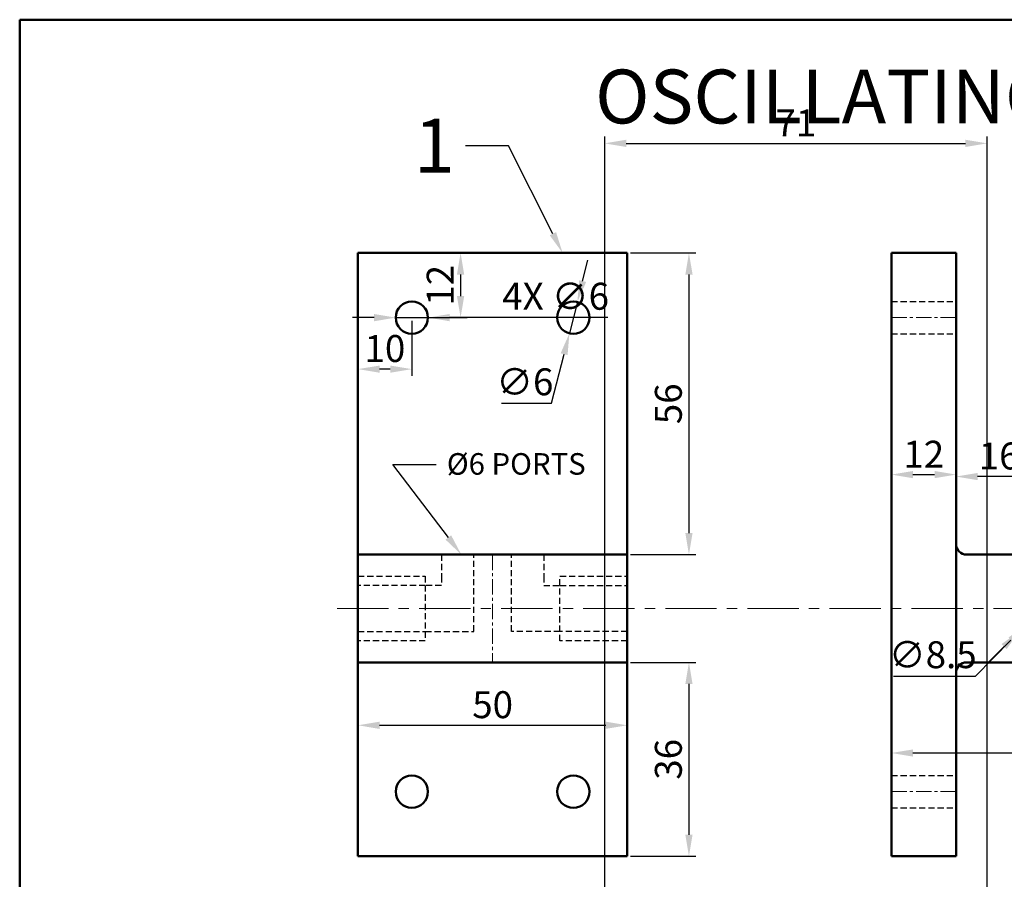
# Model space of a CAD drawing. Units: millimetres. Extents: x 24 to 508, y -182 to 223.
# Tile 2 of 6: x 24 to 207, y 63 to 223. Entities that reach past the tile are written whole.
import ezdxf
from ezdxf import colors
from ezdxf.entities.mleader import LeaderData, LeaderLine
from ezdxf.math import Vec2, Vec3

# ---------------------------------------------------------------- set-up
doc = ezdxf.new("R2010")
doc.units = ezdxf.units.MM
doc.header["$LTSCALE"] = 0.3
doc.linetypes.add('CENTER', pattern=[50.8, 31.75, -6.35, 6.35, -6.35])
doc.linetypes.add('DASHED', pattern=[19.05, 12.7, -6.35])
for name, color, linetype, lineweight in [('M-CNTR', 1, 'CENTER', 18), ('M-DIMS', 2, 'Continuous', 25), ('M-HIDN', 4, 'DASHED', 25), ('M-OUTL', 7, 'Continuous', 50), ('M-TEXT', 7, 'Continuous', 25)]:
    doc.layers.add(name, color=color, linetype=linetype, lineweight=lineweight)
doc.styles.get("Standard").update_dxf_attribs({"font": 'arial.ttf'})
doc.dimstyles.new('ISO-25', dxfattribs={"dimtxt": 5, "dimasz": 4, "dimexe": 1.25, "dimexo": 0.625, "dimtad": 1, "dimtoh": 1, "dimdec": 0, "dimtxsty": 'Standard', "dimcen": 2.5, "dimadec": 0, "dimazin": 0, "dimtfac": 1, "dimtdec": 0, "dimtmove": 0, "dimatfit": 3, "dimfxl": 1, "dimarcsym": 0})

# ---------------------------------------------------------------- blocks, each defined once
blk = doc.blocks.new('*D1')
at = {"layer": 'Defpoints', "color": 0, "ltscale": 0.3, "transparency": 16777216}
for p in [(136.55, 179.44), (136.55, 123.44), (148.01, 123.44)]:
    blk.add_point(p, dxfattribs=at)
at = {"layer": 'M-DIMS', "color": 0, "lineweight": -2, "ltscale": 0.3, "transparency": 16777216}
for p, q in [((137.17, 179.44), (149.26, 179.44)), ((148.01, 175.44), (148.01, 127.44)), ((137.17, 123.44), (149.26, 123.44))]:
    blk.add_line(p, q, dxfattribs=at)
at = {"layer": 'M-DIMS', "color": 0, "ltscale": 0.3, "transparency": 16777216}
for points in [[(147.34, 175.44), (148.68, 175.44), (148.01, 179.44)], [(147.34, 127.44), (148.68, 127.44), (148.01, 123.44)]]:
    blk.add_solid(points, dxfattribs=at)
at = {"layer": 'M-DIMS', "color": 0, "ltscale": 0.3, "transparency": 16777216, "insert": (144.83, 151.44), "char_height": 5, "attachment_point": 5, "rotation": 90}
blk.add_mtext('56', dxfattribs=at)
blk = doc.blocks.new('*D2')
at = {"layer": 'Defpoints', "color": 0, "ltscale": 0.3, "transparency": 16777216}
for p in [(136.55, 103.44), (136.55, 67.44), (148.01, 67.44)]:
    blk.add_point(p, dxfattribs=at)
at = {"layer": 'M-DIMS', "color": 0, "lineweight": -2, "ltscale": 0.3, "transparency": 16777216}
for p, q in [((137.17, 103.44), (149.26, 103.44)), ((148.01, 99.44), (148.01, 71.44)), ((137.17, 67.44), (149.26, 67.44))]:
    blk.add_line(p, q, dxfattribs=at)
at = {"layer": 'M-DIMS', "color": 0, "ltscale": 0.3, "transparency": 16777216}
for points in [[(147.34, 99.44), (148.68, 99.44), (148.01, 103.44)], [(147.34, 71.44), (148.68, 71.44), (148.01, 67.44)]]:
    blk.add_solid(points, dxfattribs=at)
at = {"layer": 'M-DIMS', "color": 0, "ltscale": 0.3, "transparency": 16777216, "insert": (144.83, 85.44), "char_height": 5, "attachment_point": 5, "rotation": 90}
blk.add_mtext('36', dxfattribs=at)
blk = doc.blocks.new('*D3')
at = {"layer": 'Defpoints', "color": 0, "ltscale": 0.3, "transparency": 16777216}
for p in [(86.55, 179.44), (96.55, 167.44), (105.6, 167.44)]:
    blk.add_point(p, dxfattribs=at)
at = {"layer": 'M-DIMS', "color": 0, "lineweight": -2, "ltscale": 0.3, "transparency": 16777216}
for p, q in [((87.17, 179.44), (106.85, 179.44)), ((105.6, 175.44), (105.6, 171.44)), ((97.17, 167.44), (106.85, 167.44))]:
    blk.add_line(p, q, dxfattribs=at)
at = {"layer": 'M-DIMS', "color": 0, "ltscale": 0.3, "transparency": 16777216}
for points in [[(104.93, 175.44), (106.27, 175.44), (105.6, 179.44)], [(104.93, 171.44), (106.27, 171.44), (105.6, 167.44)]]:
    blk.add_solid(points, dxfattribs=at)
at = {"layer": 'M-DIMS', "color": 0, "ltscale": 0.3, "transparency": 16777216, "insert": (102.46, 173.44), "char_height": 5, "attachment_point": 5, "rotation": 90}
blk.add_mtext('12', dxfattribs=at)
blk = doc.blocks.new('*D4')
at = {"layer": 'Defpoints', "color": 0, "ltscale": 0.3, "transparency": 16777216}
for p in [(86.55, 167.44), (96.55, 167.44), (86.55, 157.88)]:
    blk.add_point(p, dxfattribs=at)
at = {"layer": 'M-DIMS', "color": 0, "lineweight": -2, "ltscale": 0.3, "transparency": 16777216}
for p, q in [((86.55, 166.82), (86.55, 156.63)), ((96.55, 166.82), (96.55, 156.63)), ((92.55, 157.88), (90.55, 157.88))]:
    blk.add_line(p, q, dxfattribs=at)
at = {"layer": 'M-DIMS', "color": 0, "ltscale": 0.3, "transparency": 16777216}
for points in [[(90.55, 158.54), (90.55, 157.21), (86.55, 157.88)], [(92.55, 158.54), (92.55, 157.21), (96.55, 157.88)]]:
    blk.add_solid(points, dxfattribs=at)
at = {"layer": 'M-DIMS', "color": 0, "ltscale": 0.3, "transparency": 16777216, "insert": (91.55, 161.06), "char_height": 5, "attachment_point": 5}
blk.add_mtext('10', dxfattribs=at)
blk = doc.blocks.new('*D5')
at = {"layer": 'Defpoints', "color": 0, "ltscale": 0.3, "transparency": 16777216}
for p in [(127.29, 170.35), (125.81, 164.53)]:
    blk.add_point(p, dxfattribs=at)
at = {"layer": 'M-DIMS', "color": 0, "lineweight": -2, "ltscale": 0.3, "transparency": 16777216}
for p, q in [((128.27, 174.22), (129.26, 178.1)), ((127.29, 170.35), (125.81, 164.53)), ((122.51, 151.56), (124.82, 160.66)), ((113.17, 151.56), (122.51, 151.56))]:
    blk.add_line(p, q, dxfattribs=at)
at = {"layer": 'M-DIMS', "color": 0, "ltscale": 0.3, "transparency": 16777216}
for points in [[(127.63, 174.39), (128.92, 174.06), (127.29, 170.35)], [(124.18, 160.82), (125.47, 160.49), (125.81, 164.53)]]:
    blk.add_solid(points, dxfattribs=at)
at = {"layer": 'M-DIMS', "color": 0, "ltscale": 0.3, "transparency": 16777216, "insert": (117.53, 154.88), "char_height": 5, "attachment_point": 5}
blk.add_mtext('∅6', dxfattribs=at)
blk = doc.blocks.new('*D6')
at = {"layer": 'Defpoints', "color": 0, "ltscale": 0.3, "transparency": 16777216}
for p in [(86.55, 93.5), (136.55, 93.5), (136.55, 91.76)]:
    blk.add_point(p, dxfattribs=at)
at = {"layer": 'M-DIMS', "color": 0, "lineweight": -2, "ltscale": 0.3, "transparency": 16777216}
for p, q in [((86.55, 92.88), (86.55, 90.51)), ((90.55, 91.76), (132.55, 91.76)), ((136.55, 92.88), (136.55, 90.51))]:
    blk.add_line(p, q, dxfattribs=at)
at = {"layer": 'M-DIMS', "color": 0, "ltscale": 0.3, "transparency": 16777216}
for points in [[(90.55, 92.43), (90.55, 91.09), (86.55, 91.76)], [(132.55, 92.43), (132.55, 91.09), (136.55, 91.76)]]:
    blk.add_solid(points, dxfattribs=at)
at = {"layer": 'M-DIMS', "color": 0, "ltscale": 0.3, "transparency": 16777216, "insert": (111.55, 94.94), "char_height": 5, "attachment_point": 5}
blk.add_mtext('50', dxfattribs=at)
blk = doc.blocks.new('*D7')
at = {"layer": 'Defpoints', "color": 0, "ltscale": 0.3, "transparency": 16777216}
for p in [(185.61, 143.18), (197.61, 143.18), (197.61, 138.3)]:
    blk.add_point(p, dxfattribs=at)
at = {"layer": 'M-DIMS', "color": 0, "lineweight": -2, "ltscale": 0.3, "transparency": 16777216}
for p, q in [((185.61, 142.55), (185.61, 137.05)), ((197.61, 142.55), (197.61, 137.05)), ((189.61, 138.3), (193.61, 138.3))]:
    blk.add_line(p, q, dxfattribs=at)
at = {"layer": 'M-DIMS', "color": 0, "ltscale": 0.3, "transparency": 16777216}
for points in [[(189.61, 138.97), (189.61, 137.63), (185.61, 138.3)], [(193.61, 138.97), (193.61, 137.63), (197.61, 138.3)]]:
    blk.add_solid(points, dxfattribs=at)
at = {"layer": 'M-DIMS', "color": 0, "ltscale": 0.3, "transparency": 16777216, "insert": (191.61, 141.43), "char_height": 5, "attachment_point": 5}
blk.add_mtext('12', dxfattribs=at)
blk = doc.blocks.new('*D8')
at = {"layer": 'Defpoints', "color": 0, "ltscale": 0.3, "transparency": 16777216}
for p in [(197.61, 137.94), (197.61, 113.44), (213.61, 113.44)]:
    blk.add_point(p, dxfattribs=at)
at = {"layer": 'M-DIMS', "color": 0, "lineweight": -2, "ltscale": 0.3, "transparency": 16777216}
for p, q in [((197.61, 114.07), (197.61, 139.19)), ((213.61, 114.07), (213.61, 139.19)), ((209.61, 137.94), (201.61, 137.94))]:
    blk.add_line(p, q, dxfattribs=at)
at = {"layer": 'M-DIMS', "color": 0, "ltscale": 0.3, "transparency": 16777216}
for points in [[(201.61, 138.6), (201.61, 137.27), (197.61, 137.94)], [(209.61, 138.6), (209.61, 137.27), (213.61, 137.94)]]:
    blk.add_solid(points, dxfattribs=at)
at = {"layer": 'M-DIMS', "color": 0, "ltscale": 0.3, "transparency": 16777216, "insert": (205.61, 141.11), "char_height": 5, "attachment_point": 5}
blk.add_mtext('16', dxfattribs=at)
blk = doc.blocks.new('*D13')
at = {"layer": 'Defpoints', "color": 0, "ltscale": 0.3, "transparency": 16777216}
for p in [(247.61, 103.44), (185.61, 97.23), (247.61, 86.62)]:
    blk.add_point(p, dxfattribs=at)
at = {"layer": 'M-DIMS', "color": 0, "lineweight": -2, "ltscale": 0.3, "transparency": 16777216}
for p, q in [((247.61, 102.82), (247.61, 85.37)), ((185.61, 96.6), (185.61, 85.37)), ((189.61, 86.62), (243.61, 86.62))]:
    blk.add_line(p, q, dxfattribs=at)
at = {"layer": 'M-DIMS', "color": 0, "ltscale": 0.3, "transparency": 16777216}
for points in [[(189.61, 87.28), (189.61, 85.95), (185.61, 86.62)], [(243.61, 87.28), (243.61, 85.95), (247.61, 86.62)]]:
    blk.add_solid(points, dxfattribs=at)
at = {"layer": 'M-DIMS', "color": 0, "ltscale": 0.3, "transparency": 16777216, "insert": (216.61, 89.8), "char_height": 5, "attachment_point": 5}
blk.add_mtext('62', dxfattribs=at)
blk = doc.blocks.new('*D68')
at = {"layer": 'Defpoints', "color": 0, "ltscale": 0.3, "transparency": 16777216}
for p in [(203.36, 199.79), (132.36, 15.94), (203.36, 15.94)]:
    blk.add_point(p, dxfattribs=at)
at = {"layer": 'M-DIMS', "color": 0, "lineweight": -2, "ltscale": 0.3, "transparency": 16777216}
for p, q in [((132.36, 16.57), (132.36, 201.04)), ((136.36, 199.79), (199.36, 199.79)), ((203.36, 16.57), (203.36, 201.04))]:
    blk.add_line(p, q, dxfattribs=at)
at = {"layer": 'M-DIMS', "color": 0, "ltscale": 0.3, "transparency": 16777216}
for points in [[(136.36, 200.46), (136.36, 199.12), (132.36, 199.79)], [(199.36, 200.46), (199.36, 199.12), (203.36, 199.79)]]:
    blk.add_solid(points, dxfattribs=at)
at = {"layer": 'M-DIMS', "color": 0, "ltscale": 0.3, "transparency": 16777216, "insert": (167.86, 202.93), "char_height": 5, "attachment_point": 5}
blk.add_mtext('71', dxfattribs=at)
blk = doc.blocks.new('*D78')
at = {"layer": 'Defpoints', "color": 0, "ltscale": 0.3, "transparency": 16777216}
for p in [(93.55, 167.44), (99.55, 167.44)]:
    blk.add_point(p, dxfattribs=at)
at = {"layer": 'M-DIMS', "color": 0, "lineweight": -2, "ltscale": 0.3, "transparency": 16777216}
for p, q in [((89.55, 167.44), (85.55, 167.44)), ((93.55, 167.44), (99.55, 167.44)), ((112.93, 167.44), (103.55, 167.44)), ((132.95, 167.44), (112.93, 167.44))]:
    blk.add_line(p, q, dxfattribs=at)
at = {"layer": 'M-DIMS', "color": 0, "ltscale": 0.3, "transparency": 16777216}
for points in [[(89.55, 168.11), (89.55, 166.77), (93.55, 167.44)], [(103.55, 168.11), (103.55, 166.77), (99.55, 167.44)]]:
    blk.add_solid(points, dxfattribs=at)
at = {"layer": 'M-DIMS', "color": 0, "ltscale": 0.3, "transparency": 16777216, "insert": (123.25, 170.76), "char_height": 5, "attachment_point": 5}
blk.add_mtext('4X ∅6', dxfattribs=at)
blk = doc.blocks.new('*D79')
at = {"layer": 'Defpoints', "color": 0, "ltscale": 0.3, "transparency": 16777216}
for p in [(217.85, 117.68), (209.36, 109.2)]:
    blk.add_point(p, dxfattribs=at)
at = {"layer": 'M-DIMS', "color": 0, "lineweight": -2, "ltscale": 0.3, "transparency": 16777216}
for p, q in [((223.51, 123.34), (220.68, 120.51)), ((236.69, 123.34), (223.51, 123.34)), ((209.36, 109.2), (217.85, 117.68)), ((206.53, 106.37), (203.7, 103.55))]:
    blk.add_line(p, q, dxfattribs=at)
at = {"layer": 'M-DIMS', "color": 0, "ltscale": 0.3, "transparency": 16777216}
for points in [[(220.21, 120.98), (221.15, 120.04), (217.85, 117.68)], [(206.06, 106.84), (207, 105.9), (209.36, 109.2)]]:
    blk.add_solid(points, dxfattribs=at)
at = {"layer": 'M-DIMS', "color": 0, "ltscale": 0.3, "transparency": 16777216, "insert": (230.41, 126.65), "char_height": 5, "attachment_point": 5}
blk.add_mtext('∅12', dxfattribs=at)
blk = doc.blocks.new('*D80')
at = {"layer": 'Defpoints', "color": 0, "ltscale": 0.3, "transparency": 16777216}
for p in [(216.59, 116.46), (210.62, 110.42)]:
    blk.add_point(p, dxfattribs=at)
at = {"layer": 'M-DIMS', "color": 0, "lineweight": -2, "ltscale": 0.3, "transparency": 16777216}
for p, q in [((219.41, 119.31), (222.22, 122.15)), ((216.59, 116.46), (210.62, 110.42)), ((201.21, 100.9), (207.81, 107.57)), ((186, 100.9), (201.21, 100.9))]:
    blk.add_line(p, q, dxfattribs=at)
at = {"layer": 'M-DIMS', "color": 0, "ltscale": 0.3, "transparency": 16777216}
for points in [[(218.93, 119.78), (219.88, 118.84), (216.59, 116.46)], [(207.33, 108.04), (208.28, 107.11), (210.62, 110.42)]]:
    blk.add_solid(points, dxfattribs=at)
at = {"layer": 'M-DIMS', "color": 0, "ltscale": 0.3, "transparency": 16777216, "insert": (193.29, 104.22), "char_height": 5, "attachment_point": 5}
blk.add_mtext('∅8.5', dxfattribs=at)

msp = doc.modelspace()

# ---------------------------------------------------------------- linework, layer by layer
at = {"layer": 'M-CNTR', "ltscale": 0.3}
for p, q in [((185.6065, 167.4403), (197.6065, 167.4403)), ((111.5473, 123.4403), (111.5473, 103.4403)), ((185.6065, 79.4403), (197.6065, 79.4403))]:
    msp.add_line(p, q, dxfattribs=at)
at = {"layer": 'M-CNTR'}
msp.add_line((82.668, 113.4403), (347.6065, 113.4403), dxfattribs=at)
at = {"layer": 'M-HIDN', "ltscale": 0.3}
for p, q in [((185.6065, 170.4403), (197.6065, 170.4403)), ((185.6065, 164.4403), (197.6065, 164.4403)), ((185.6065, 82.4403), (197.6065, 82.4403)), ((185.6065, 76.4403), (197.6065, 76.4403))]:
    msp.add_line(p, q, dxfattribs=at)
for points in [[(86.5473, 109.1903), (99.0473, 109.1903), (108.0473, 109.1903), (108.0473, 119.4403), (108.0473, 123.4403)], [(102.0473, 123.4403), (102.0473, 119.4403), (102.0473, 117.6903), (99.0473, 117.6903), (86.5473, 117.6903)], [(136.5473, 109.1903), (124.0473, 109.1903), (115.0473, 109.1903), (115.0473, 119.4403), (115.0473, 123.4403)], [(121.0473, 123.4403), (121.0473, 119.4403), (121.0473, 117.6903), (124.0473, 117.6903), (136.5473, 117.6903)], [(86.5473, 119.4403), (99.0473, 119.4403), (99.0473, 107.4403), (86.5473, 107.4403)], [(136.5473, 107.4403), (124.0473, 107.4403), (124.0473, 119.4403), (136.5473, 119.4403)]]:
    msp.add_lwpolyline(points, dxfattribs=at)
at = {"layer": 'M-OUTL'}
for p, q in [((86.5473, 67.4403), (86.5473, 179.4403)), ((86.5473, 179.4403), (136.5473, 179.4403)), ((136.5473, 179.4403), (136.5473, 67.4403)), ((185.6065, 179.4403), (185.6065, 67.4403)), ((197.6065, 179.4403), (185.6065, 179.4403)), ((197.6065, 101.4403), (197.6065, 179.4403)), ((136.5473, 123.4403), (86.5473, 123.4403)), ((346.4065, 123.4403), (199.6065, 123.4403)), ((136.5473, 103.4403), (86.5473, 103.4403)), ((346.4065, 103.4403), (199.6065, 103.4403)), ((197.6065, 67.4403), (197.6065, 101.4403)), ((136.5473, 67.4403), (86.5473, 67.4403)), ((185.6065, 67.4403), (197.6065, 67.4403))]:
    msp.add_line(p, q, dxfattribs=at)
at = {"layer": 'M-OUTL', "ltscale": 0.3}
msp.add_lwpolyline([(23.7253, 222.7463), (508.4225, 222.7463), (508.4225, -181.5799), (23.7253, -181.5799)], close=True, dxfattribs=at)
for centre in [(96.5473, 167.4403), (126.5473, 167.4403), (96.5473, 79.4403), (126.5473, 79.4403)]:
    msp.add_circle(centre, 3, dxfattribs=at)
at = {"layer": 'M-OUTL'}
for centre, start, end in [((199.6065, 125.4403), 180, 270), ((199.6065, 101.4403), 90, 180)]:
    msp.add_arc(centre, 2, start, end, dxfattribs=at)

# ---------------------------------------------------------------- texts
at = {"layer": 'M-TEXT', "ltscale": 0.3, "insert": (130.5797, 213.4834), "char_height": 10, "attachment_point": 1}
msp.add_mtext_dynamic_manual_height_columns('OSCILLATING PUMP ASSEMBLY COMPONENTS', width=327.515557, gutter_width=12.5, heights=[0], dxfattribs=at)

# ---------------------------------------------------------------- dimensions: what is measured, and where the dimension line sits
at = {"layer": 'M-DIMS', "ltscale": 0.3}
for base, p1, p2, override, picture, middle in [((203.3582, 199.7903), (132.3582, 15.9426), (203.3582, 15.9426), {"dimdec": 0, "dimlfac": 1, "dimrnd": 0, "dimzin": 0, "dimdsep": 46, "dimlunit": 2}, '*D68', (167.8582, 202.9256)), ((86.5473, 157.8777), (96.5473, 167.4403), (86.5473, 167.4403), {"dimclrd": 0, "dimclre": 0, "dimclrt": 0}, '*D4', (91.5473, 161.0556)), ((197.6065, 138.2993), (185.6065, 143.1763), (197.6065, 143.1763), {"dimclrd": 0, "dimclre": 0, "dimclrt": 0}, '*D7', (191.6065, 141.4345)), ((197.6065, 137.9361), (213.6065, 113.4403), (197.6065, 113.4403), {"dimclrd": 0, "dimclre": 0, "dimclrt": 0}, '*D8', (205.6065, 141.114)), ((247.6065, 86.6173), (185.6065, 97.2279), (247.6065, 103.4403), {"dimclrd": 0, "dimclre": 0, "dimclrt": 0}, '*D13', (216.6065, 89.7952)), ((136.5473, 91.7587), (86.5473, 93.5005), (136.5473, 93.5005), {"dimclrd": 0, "dimclre": 0, "dimclrt": 0}, '*D6', (111.5473, 94.9366))]:
    dim = msp.add_linear_dim(base=base, p1=p1, p2=p2, dimstyle='ISO-25', override=override, dxfattribs=at)
    dim.commit()
    dim.dimension.update_dxf_attribs({"geometry": picture, "text_midpoint": middle})
for base, p1, p2, picture, middle in [((105.5984, 167.4403), (86.5473, 179.4403), (96.5473, 167.4403), '*D3', (102.4632, 173.4403)), ((148.01, 123.4403), (136.5473, 179.4403), (136.5473, 123.4403), '*D1', (144.8321, 151.4403)), ((148.01, 67.4403), (136.5473, 103.4403), (136.5473, 67.4403), '*D2', (144.8304, 85.4403))]:
    dim = msp.add_linear_dim(base=base, p1=p1, p2=p2, angle=90, dimstyle='ISO-25', override={"dimclrd": 0, "dimclre": 0, "dimclrt": 0}, dxfattribs=at)
    dim.commit()
    dim.dimension.update_dxf_attribs({"geometry": picture, "text_midpoint": middle})
dim = msp.add_diameter_dim_2p(p1=(93.5473, 167.4407), p2=(99.5473, 167.44), text='4X <>', dimstyle='ISO-25', override={"dimdec": 0, "dimlfac": 1, "dimrnd": 0, "dimzin": 0, "dimdsep": 46, "dimlunit": 2}, dxfattribs=at)
dim.commit()
dim.dimension.update_dxf_attribs({"geometry": '*D78', "text_midpoint": (112.9327, 167.4385)})
dim = msp.add_diameter_dim_2p(p1=(127.2869, 170.3477), p2=(125.8077, 164.5329), dimstyle='ISO-25', override={"dimclrd": 0, "dimclre": 0, "dimclrt": 0}, dxfattribs=at)
dim.commit()
dim.dimension.update_dxf_attribs({"geometry": '*D5', "text_midpoint": (117.5257, 154.8784)})
for p1, p2, override, picture, middle in [((209.3619, 109.1996), (217.8511, 117.6811), {"dimdec": 0, "dimlfac": 1, "dimrnd": 0, "dimzin": 0, "dimdsep": 46, "dimlunit": 2}, '*D79', (230.4111, 123.3353)), ((216.5948, 116.4623), (210.6182, 110.4184), {"dimdec": 1, "dimlfac": 1, "dimrnd": 0, "dimzin": 0, "dimdsep": 46, "dimlunit": 2}, '*D80', (193.2911, 100.9006))]:
    dim = msp.add_diameter_dim_2p(p1=p1, p2=p2, dimstyle='ISO-25', override=override, dxfattribs=at)
    dim.commit()
    dim.dimension.update_dxf_attribs({"geometry": picture, "text_midpoint": middle, "dimtype": 163})

# ---------------------------------------------------------------- leaders
ml = msp.add_multileader_mtext('Standard', dxfattribs=at)
ml.set_content('1', color=256)
ml.set_leader_properties()
ml.build(insert=Vec2(0, 0))
ctx = ml.context
ctx.base_point, ctx.char_height, ctx.plane_origin = Vec3(98.8435, 199.3599), 10, Vec3(124.5431, 179.4403)
ctx.text_align_type = 2
notes = []
notes.append((ctx, [(0, (1, 1, 0), (114.527, 199.3599), (-1, 0), 8, [(0, [(124.5431, 179.4403)], 0, [])])]))
ctx.mtext.insert, ctx.mtext.alignment, ctx.mtext.flow_direction = Vec3(104.527, 204.3599), 3, 5
ml = msp.add_multileader_mtext('Standard', dxfattribs=at)
ml.set_content('%%C6 PORTS', color=256)
ml.set_leader_properties()
ml.build(insert=Vec2(0, 0))
ctx = ml.context
ctx.base_point, ctx.plane_origin = Vec3(101.0458, 140.2014), Vec3(105.7424, 123.4403)
notes.append((ctx, [(0, (1, 1, 0), (93.0458, 140.2014), (1, 0), 8, [(0, [(105.7424, 123.4403)], 0, [])])]))
ctx.mtext.insert, ctx.mtext.flow_direction = Vec3(103.0458, 142.2819), 5
for ctx, leaders in notes:
    for number, flags, end, landing, length, lines in leaders:
        leader = LeaderData()
        leader.index, (leader.has_last_leader_line, leader.has_dogleg_vector, leader.attachment_direction) = number, flags
        leader.last_leader_point, leader.dogleg_vector, leader.dogleg_length = Vec3(end), Vec3(landing), length
        for number, points, colour, breaks in lines:
            line = LeaderLine()
            line.index, line.vertices, line.color, line.breaks = number, Vec3.list(points), colors.encode_raw_color(colour), breaks
            leader.lines.append(line)
        ctx.leaders.append(leader)

doc.saveas('drawing.dxf')
